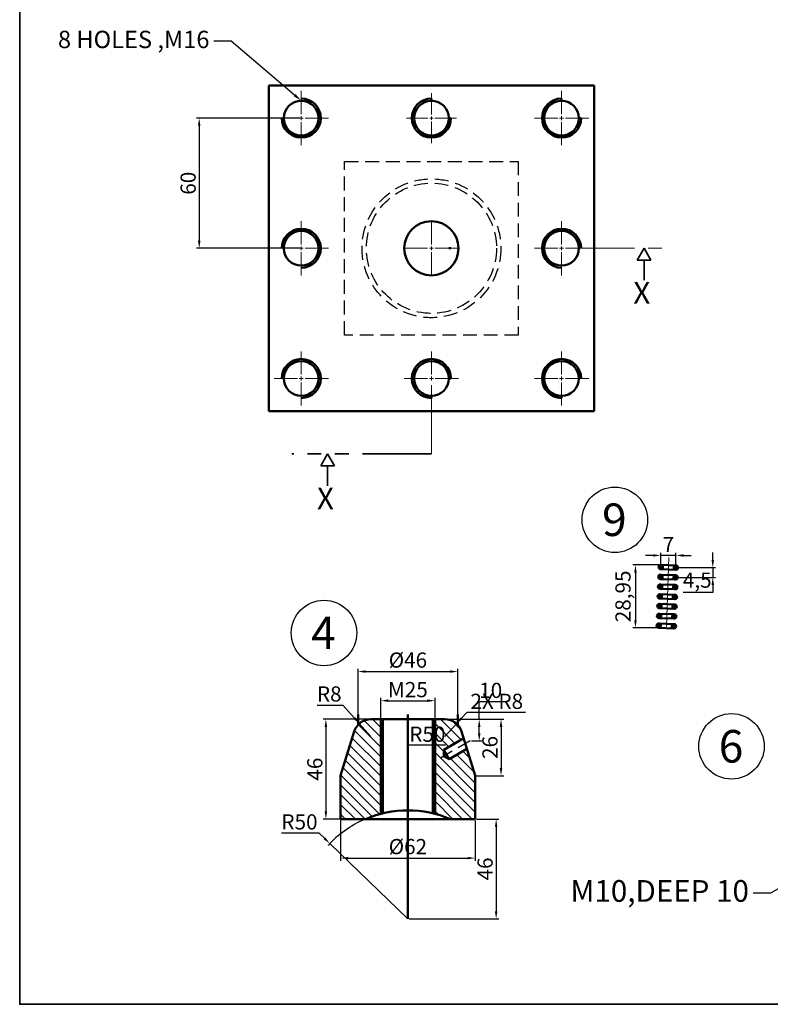
# Model space of a CAD drawing. Units: millimetres. Extents: x -5 to 1372, y -339 to 395.
# Tile 1 of 6: x -5 to 341, y -339 to 114. Entities that reach past the tile are written whole.
import ezdxf
from ezdxf import colors
from ezdxf.entities.mleader import LeaderData, LeaderLine
from ezdxf.math import Vec2, Vec3

# ---------------------------------------------------------------- set-up
doc = ezdxf.new("R2010")
doc.units = ezdxf.units.MM
for name, pattern in [('CENTER', [50.8, 31.75, -6.35, 6.35, -6.35]), ('HIDDEN', [9.525, 6.35, -3.175]), ('PHANTOM', [63.5, 31.75, -6.35, 6.35, -6.35, 6.35, -6.35])]:
    doc.linetypes.add(name, pattern=pattern)
for name, color, linetype, lineweight in [('M-CNTR', 1, 'CENTER', 18), ('M-DIMS', 2, 'Continuous', 25), ('M-HATC', 8, 'Continuous', 18), ('M-HIDN', 6, 'HIDDEN', 25), ('M-OUTL', 7, 'Continuous', 50), ('M-SECT', 4, 'PHANTOM', 35), ('M-TEXT', 3, 'Continuous', 25), ('M-TTLB', 7, 'Continuous', 35)]:
    doc.layers.add(name, color=color, linetype=linetype, lineweight=lineweight)
doc.styles.get("Standard").update_dxf_attribs({"font": 'arial.ttf'})
doc.dimstyles.new('ISO-25', dxfattribs={"dimtxt": 7, "dimasz": 3.5, "dimexe": 1.25, "dimexo": 0.625, "dimtad": 1, "dimtoh": 1, "dimtxsty": 'Standard', "dimcen": 2.5, "dimadec": 0, "dimazin": 0, "dimtfac": 1, "dimtmove": 0, "dimatfit": 3, "dimfxl": 1, "dimarcsym": 0})
pattern_1 = [(133, (-372.26105, -76.62878), (-0.2322048, -0.21653448), [])]
pattern_2 = [(133, (-372.4181, -81.12604), (-0.2322048, -0.21653448), [])]
pattern_3 = [(133, (-372.57515, -85.6233), (-0.2322048, -0.21653448), [])]
pattern_4 = [(133, (-372.7322, -90.12055), (-0.2322048, -0.21653448), [])]
pattern_5 = [(133, (-372.88924, -94.6178), (-0.2322048, -0.21653448), [])]
pattern_6 = [(133, (-373.0463, -99.11507), (-0.2322048, -0.21653448), [])]
pattern_7 = [(133, (-373.20334, -103.61233), (-0.2322048, -0.21653448), [])]

# ---------------------------------------------------------------- blocks, each defined once
blk = doc.blocks.new('*U17')
at = {"layer": 'M-CNTR', "color": 0, "transparency": 16777216}
for p, q in [((0, 1.8), (0, 12.5)), ((-12.5, 0), (-1.8, 0)), ((1.8, 0), (12.5, 0)), ((0, -12.5), (0, -1.8))]:
    blk.add_line(p, q, dxfattribs=at)
at = {"layer": 'M-CNTR', "color": 0, "linetype": 'Continuous', "transparency": 16777216}
for p, q in [((-0.9, 0), (0.9, 0)), ((0, -0.9), (0, 0.9))]:
    blk.add_line(p, q, dxfattribs=at)
blk = doc.blocks.new('*U18')
at = {"layer": 'M-CNTR', "color": 0, "transparency": 16777216}
for p, q in [((0, 1.8), (0, 12.5)), ((-12.5, 0), (-1.8, 0)), ((1.8, 0), (12.5, 0)), ((0, -34.79), (0, -1.8))]:
    blk.add_line(p, q, dxfattribs=at)
at = {"layer": 'M-CNTR', "color": 0, "linetype": 'Continuous', "transparency": 16777216}
for p, q in [((-0.9, 0), (0.9, 0)), ((0, -0.9), (0, 0.9))]:
    blk.add_line(p, q, dxfattribs=at)
blk = doc.blocks.new('*U19')
at = {"layer": 'M-CNTR', "color": 0, "transparency": 16777216}
for p, q in [((0, 1.8), (0, 12.5)), ((-12.5, 0), (-1.8, 0)), ((1.8, 0), (47.58, 0)), ((0, -12.5), (0, -1.8))]:
    blk.add_line(p, q, dxfattribs=at)
at = {"layer": 'M-CNTR', "color": 0, "linetype": 'Continuous', "transparency": 16777216}
for p, q in [((-0.9, 0), (0.9, 0)), ((0, -0.9), (0, 0.9))]:
    blk.add_line(p, q, dxfattribs=at)
blk = doc.blocks.new('*U20')
at = {"layer": 'M-CNTR', "color": 0, "transparency": 16777216}
for p, q in [((0, 1.8), (0, 12.5)), ((-12.5, 0), (-1.8, 0)), ((1.8, 0), (12.5, 0)), ((0, -12.5), (0, -1.8))]:
    blk.add_line(p, q, dxfattribs=at)
at = {"layer": 'M-CNTR', "color": 0, "linetype": 'Continuous', "transparency": 16777216}
for p, q in [((-0.9, 0), (0.9, 0)), ((0, -0.9), (0, 0.9))]:
    blk.add_line(p, q, dxfattribs=at)
blk = doc.blocks.new('*U21')
at = {"layer": 'M-CNTR', "color": 0, "transparency": 16777216}
for p, q in [((0, 1.8), (0, 12.5)), ((-12.5, 0), (-1.8, 0)), ((1.8, 0), (12.5, 0)), ((0, -12.5), (0, -1.8))]:
    blk.add_line(p, q, dxfattribs=at)
at = {"layer": 'M-CNTR', "color": 0, "linetype": 'Continuous', "transparency": 16777216}
for p, q in [((-0.9, 0), (0.9, 0)), ((0, -0.9), (0, 0.9))]:
    blk.add_line(p, q, dxfattribs=at)
blk = doc.blocks.new('*U22')
at = {"layer": 'M-CNTR', "color": 0, "transparency": 16777216}
for p, q in [((0, 1.8), (0, 12.5)), ((-12.5, 0), (-1.8, 0)), ((1.8, 0), (12.5, 0)), ((0, -12.5), (0, -1.8))]:
    blk.add_line(p, q, dxfattribs=at)
at = {"layer": 'M-CNTR', "color": 0, "linetype": 'Continuous', "transparency": 16777216}
for p, q in [((-0.9, 0), (0.9, 0)), ((0, -0.9), (0, 0.9))]:
    blk.add_line(p, q, dxfattribs=at)
blk = doc.blocks.new('*U23')
at = {"layer": 'M-CNTR', "color": 0, "transparency": 16777216}
for p, q in [((0, 1.6), (0, 11.5)), ((-11.5, 0), (-1.6, 0)), ((1.6, 0), (11.5, 0)), ((0, -11.5), (0, -1.6))]:
    blk.add_line(p, q, dxfattribs=at)
at = {"layer": 'M-CNTR', "color": 0, "linetype": 'Continuous', "transparency": 16777216}
for p, q in [((-0.8, 0), (0.8, 0)), ((0, -0.8), (0, 0.8))]:
    blk.add_line(p, q, dxfattribs=at)
blk = doc.blocks.new('*U24')
at = {"layer": 'M-CNTR', "color": 0, "transparency": 16777216}
for p, q in [((0, 1.8), (0, 12.5)), ((-12.5, 0), (-1.8, 0)), ((1.8, 0), (12.5, 0)), ((0, -12.5), (0, -1.8))]:
    blk.add_line(p, q, dxfattribs=at)
at = {"layer": 'M-CNTR', "color": 0, "linetype": 'Continuous', "transparency": 16777216}
for p, q in [((-0.9, 0), (0.9, 0)), ((0, -0.9), (0, 0.9))]:
    blk.add_line(p, q, dxfattribs=at)
blk = doc.blocks.new('*U25')
at = {"layer": 'M-CNTR', "color": 0, "transparency": 16777216}
for p, q in [((0, 1.8), (0, 12.5)), ((-12.5, 0), (-1.8, 0)), ((1.8, 0), (12.5, 0)), ((0, -12.5), (0, -1.8))]:
    blk.add_line(p, q, dxfattribs=at)
at = {"layer": 'M-CNTR', "color": 0, "linetype": 'Continuous', "transparency": 16777216}
for p, q in [((-0.9, 0), (0.9, 0)), ((0, -0.9), (0, 0.9))]:
    blk.add_line(p, q, dxfattribs=at)
blk = doc.blocks.new('*D26')
at = {"layer": 'Defpoints', "color": 0, "transparency": 16777216}
for p in [(124.85, 69.06), (77.81, 9.06), (124.85, 9.06)]:
    blk.add_point(p, dxfattribs=at)
at = {"layer": 'M-DIMS', "color": 0, "lineweight": -2, "transparency": 16777216}
for p, q in [((124.23, 69.06), (76.56, 69.06)), ((77.81, 65.56), (77.81, 12.56)), ((124.23, 9.06), (76.56, 9.06))]:
    blk.add_line(p, q, dxfattribs=at)
at = {"layer": 'M-DIMS', "color": 0, "transparency": 16777216}
for points in [[(77.22, 65.56), (78.39, 65.56), (77.81, 69.06)], [(77.22, 12.56), (78.39, 12.56), (77.81, 9.06)]]:
    blk.add_solid(points, dxfattribs=at)
at = {"layer": 'M-DIMS', "color": 0, "transparency": 16777216, "insert": (73.61, 39.06), "char_height": 7, "attachment_point": 5, "rotation": 90}
blk.add_mtext('60', dxfattribs=at)
blk = doc.blocks.new('*D68')
at = {"layer": 'Defpoints', "color": 0, "transparency": 16777216}
for p in [(138.04, -265.26), (174.01, -299.99)]:
    blk.add_point(p, dxfattribs=at)
at = {"layer": 'M-DIMS', "color": 0, "lineweight": -2, "transparency": 16777216}
for p, q in [((115.68, -260.4), (133, -260.4)), ((133, -260.4), (135.52, -262.83)), ((174.01, -299.99), (138.04, -265.26))]:
    blk.add_line(p, q, dxfattribs=at)
blk.add_arc((174.01, -299.99), 50, 113.7901, 137.4421, dxfattribs=at)
at = {"layer": 'M-DIMS', "color": 0, "transparency": 16777216}
blk.add_solid([(135.93, -262.41), (135.12, -263.25), (138.04, -265.26)], dxfattribs=at)
at = {"layer": 'M-DIMS', "color": 0, "transparency": 16777216, "insert": (124.03, -256.2), "char_height": 7, "attachment_point": 5}
blk.add_mtext('R50', dxfattribs=at)
blk = doc.blocks.new('*D69')
at = {"layer": 'Defpoints', "color": 0, "transparency": 16777216}
for p in [(156.92, -207.99), (136.21, -253.99), (154.42, -253.99)]:
    blk.add_point(p, dxfattribs=at)
at = {"layer": 'M-DIMS', "color": 0, "lineweight": -2, "transparency": 16777216}
for p, q in [((156.3, -207.99), (134.96, -207.99)), ((136.21, -211.49), (136.21, -250.49)), ((153.79, -253.99), (134.96, -253.99))]:
    blk.add_line(p, q, dxfattribs=at)
at = {"layer": 'M-DIMS', "color": 0, "transparency": 16777216}
for points in [[(135.62, -211.49), (136.79, -211.49), (136.21, -207.99)], [(135.62, -250.49), (136.79, -250.49), (136.21, -253.99)]]:
    blk.add_solid(points, dxfattribs=at)
at = {"layer": 'M-DIMS', "color": 0, "transparency": 16777216, "insert": (132.01, -230.99), "char_height": 7, "attachment_point": 5, "rotation": 90}
blk.add_mtext('46', dxfattribs=at)
blk = doc.blocks.new('*D70')
at = {"layer": 'Defpoints', "color": 0, "transparency": 16777216}
for p in [(186.51, -199.43), (161.51, -207.99), (186.51, -207.99)]:
    blk.add_point(p, dxfattribs=at)
at = {"layer": 'M-DIMS', "color": 0, "lineweight": -2, "transparency": 16777216}
for p, q in [((161.51, -207.36), (161.51, -198.18)), ((165.01, -199.43), (183.01, -199.43)), ((186.51, -207.36), (186.51, -198.18))]:
    blk.add_line(p, q, dxfattribs=at)
at = {"layer": 'M-DIMS', "color": 0, "transparency": 16777216}
for points in [[(165.01, -198.84), (165.01, -200.01), (161.51, -199.43)], [(183.01, -198.84), (183.01, -200.01), (186.51, -199.43)]]:
    blk.add_solid(points, dxfattribs=at)
at = {"layer": 'M-DIMS', "color": 0, "transparency": 16777216, "insert": (174.01, -195.23), "char_height": 7, "attachment_point": 5}
blk.add_mtext('M25', dxfattribs=at)
blk = doc.blocks.new('*D71')
at = {"layer": 'Defpoints', "color": 0, "transparency": 16777216}
for p in [(191.1, -207.99), (205.01, -233.99), (216.94, -233.99)]:
    blk.add_point(p, dxfattribs=at)
at = {"layer": 'M-DIMS', "color": 0, "lineweight": -2, "transparency": 16777216}
for p, q in [((191.73, -207.99), (218.19, -207.99)), ((216.94, -211.49), (216.94, -230.49)), ((205.64, -233.99), (218.19, -233.99))]:
    blk.add_line(p, q, dxfattribs=at)
at = {"layer": 'M-DIMS', "color": 0, "transparency": 16777216}
for points in [[(216.35, -211.49), (217.52, -211.49), (216.94, -207.99)], [(216.35, -230.49), (217.52, -230.49), (216.94, -233.99)]]:
    blk.add_solid(points, dxfattribs=at)
at = {"layer": 'M-DIMS', "color": 0, "transparency": 16777216, "insert": (212.74, -220.99), "char_height": 7, "attachment_point": 5, "rotation": 90}
blk.add_mtext('26', dxfattribs=at)
blk = doc.blocks.new('*D72')
at = {"layer": 'Defpoints', "color": 0, "transparency": 16777216}
for p in [(202.74, -207.99), (202.74, -217.99), (206.89, -217.99)]:
    blk.add_point(p, dxfattribs=at)
at = {"layer": 'M-DIMS', "color": 0, "lineweight": -2, "transparency": 16777216}
for p, q in [((206.89, -207.99), (206.89, -199.79)), ((206.89, -199.79), (216.86, -199.79)), ((203.36, -207.99), (208.14, -207.99)), ((206.89, -214.49), (206.89, -211.49)), ((203.36, -217.99), (208.14, -217.99))]:
    blk.add_line(p, q, dxfattribs=at)
at = {"layer": 'M-DIMS', "color": 0, "transparency": 16777216}
for points in [[(206.3, -211.49), (207.47, -211.49), (206.89, -207.99)], [(206.3, -214.49), (207.47, -214.49), (206.89, -217.99)]]:
    blk.add_solid(points, dxfattribs=at)
at = {"layer": 'M-DIMS', "color": 0, "transparency": 16777216, "insert": (212.18, -195.59), "char_height": 7, "attachment_point": 5}
blk.add_mtext('10', dxfattribs=at)
blk = doc.blocks.new('*D73')
at = {"layer": 'Defpoints', "color": 0, "transparency": 16777216}
for p in [(143.01, -253.99), (205.01, -253.99), (205.01, -271.98)]:
    blk.add_point(p, dxfattribs=at)
at = {"layer": 'M-DIMS', "color": 0, "lineweight": -2, "transparency": 16777216}
for p, q in [((143.01, -254.61), (143.01, -273.23)), ((205.01, -254.61), (205.01, -273.23)), ((146.51, -271.98), (201.51, -271.98))]:
    blk.add_line(p, q, dxfattribs=at)
at = {"layer": 'M-DIMS', "color": 0, "transparency": 16777216}
for points in [[(146.51, -271.4), (146.51, -272.56), (143.01, -271.98)], [(201.51, -271.4), (201.51, -272.56), (205.01, -271.98)]]:
    blk.add_solid(points, dxfattribs=at)
at = {"layer": 'M-DIMS', "color": 0, "transparency": 16777216, "insert": (174.01, -267.58), "char_height": 7, "attachment_point": 5}
blk.add_mtext('%%C62', dxfattribs=at)
blk = doc.blocks.new('*D74')
at = {"layer": 'Defpoints', "color": 0, "transparency": 16777216}
for p in [(197.01, -186.01), (151.01, -207.99), (197.01, -207.99)]:
    blk.add_point(p, dxfattribs=at)
at = {"layer": 'M-DIMS', "color": 0, "lineweight": -2, "transparency": 16777216}
for p, q in [((151.01, -207.36), (151.01, -184.76)), ((154.51, -186.01), (193.51, -186.01)), ((197.01, -207.36), (197.01, -184.76))]:
    blk.add_line(p, q, dxfattribs=at)
at = {"layer": 'M-DIMS', "color": 0, "transparency": 16777216}
for points in [[(154.51, -185.42), (154.51, -186.59), (151.01, -186.01)], [(193.51, -185.42), (193.51, -186.59), (197.01, -186.01)]]:
    blk.add_solid(points, dxfattribs=at)
at = {"layer": 'M-DIMS', "color": 0, "transparency": 16777216, "insert": (174.01, -181.61), "char_height": 7, "attachment_point": 5}
blk.add_mtext('%%C46', dxfattribs=at)
blk = doc.blocks.new('*D75')
at = {"layer": 'Defpoints', "color": 0, "transparency": 16777216}
for p in [(151.62, -210), (156.92, -215.99)]:
    blk.add_point(p, dxfattribs=at)
at = {"layer": 'M-DIMS', "color": 0, "lineweight": -2, "transparency": 16777216}
for p, q in [((132.11, -201.43), (144.04, -201.43)), ((144.04, -201.43), (149.3, -207.37)), ((156.92, -215.99), (151.62, -210))]:
    blk.add_line(p, q, dxfattribs=at)
at = {"layer": 'M-DIMS', "color": 0, "transparency": 16777216}
blk.add_solid([(149.73, -206.99), (148.86, -207.76), (151.62, -210)], dxfattribs=at)
at = {"layer": 'M-DIMS', "color": 0, "transparency": 16777216, "insert": (137.76, -197.24), "char_height": 7, "attachment_point": 5}
blk.add_mtext('R8', dxfattribs=at)
blk = doc.blocks.new('*D76')
at = {"layer": 'Defpoints', "color": 0, "transparency": 16777216}
for p in [(205.01, -253.99), (174.01, -299.99), (214.69, -299.99)]:
    blk.add_point(p, dxfattribs=at)
at = {"layer": 'M-DIMS', "color": 0, "lineweight": -2, "transparency": 16777216}
for p, q in [((205.64, -253.99), (215.94, -253.99)), ((214.69, -257.49), (214.69, -296.49)), ((174.64, -299.99), (215.94, -299.99))]:
    blk.add_line(p, q, dxfattribs=at)
at = {"layer": 'M-DIMS', "color": 0, "transparency": 16777216}
for points in [[(214.11, -257.49), (215.27, -257.49), (214.69, -253.99)], [(214.11, -296.49), (215.27, -296.49), (214.69, -299.99)]]:
    blk.add_solid(points, dxfattribs=at)
at = {"layer": 'M-DIMS', "color": 0, "transparency": 16777216, "insert": (210.49, -276.99), "char_height": 7, "attachment_point": 5, "rotation": 90}
blk.add_mtext('46', dxfattribs=at)
blk = doc.blocks.new('*D87')
at = {"layer": 'Defpoints', "color": 0, "transparency": 16777216}
for p in [(290.59, -132.49), (290.59, -137.86), (297.59, -138.1)]:
    blk.add_point(p, dxfattribs=at)
at = {"layer": 'M-DIMS', "color": 0, "lineweight": -2, "transparency": 16777216}
for p, q in [((290.59, -137.24), (290.59, -131.24)), ((297.59, -137.48), (297.59, -131.24)), ((287.09, -132.49), (283.59, -132.49)), ((297.59, -132.49), (290.59, -132.49)), ((301.09, -132.49), (304.59, -132.49))]:
    blk.add_line(p, q, dxfattribs=at)
at = {"layer": 'M-DIMS', "color": 0, "transparency": 16777216}
for points in [[(287.09, -131.91), (287.09, -133.07), (290.59, -132.49)], [(301.09, -131.91), (301.09, -133.07), (297.59, -132.49)]]:
    blk.add_solid(points, dxfattribs=at)
at = {"layer": 'M-DIMS', "color": 0, "transparency": 16777216, "insert": (294.09, -128.37), "char_height": 7, "attachment_point": 5}
blk.add_mtext('7', dxfattribs=at)
blk = doc.blocks.new('*D88')
at = {"layer": 'Defpoints', "color": 0, "transparency": 16777216}
for p in [(297.59, -138.1), (297.43, -142.6), (314.55, -142.6)]:
    blk.add_point(p, dxfattribs=at)
at = {"layer": 'M-DIMS', "color": 0, "lineweight": -2, "transparency": 16777216}
for p, q in [((314.55, -134.6), (314.55, -131.1)), ((298.22, -138.1), (315.8, -138.1)), ((314.55, -138.1), (314.55, -142.6)), ((298.06, -142.6), (315.8, -142.6)), ((314.55, -149.6), (300.85, -149.6)), ((314.55, -146.1), (314.55, -149.6))]:
    blk.add_line(p, q, dxfattribs=at)
at = {"layer": 'M-DIMS', "color": 0, "transparency": 16777216}
for points in [[(313.97, -134.6), (315.13, -134.6), (314.55, -138.1)], [(313.97, -146.1), (315.13, -146.1), (314.55, -142.6)]]:
    blk.add_solid(points, dxfattribs=at)
at = {"layer": 'M-DIMS', "color": 0, "transparency": 16777216, "insert": (307.39, -144.78), "char_height": 7, "attachment_point": 5}
blk.add_mtext('4,5', dxfattribs=at)
blk = doc.blocks.new('*D89')
at = {"layer": 'Defpoints', "color": 0, "transparency": 16777216}
for p in [(290.36, -136.89), (278.91, -165.83), (289.35, -165.83)]:
    blk.add_point(p, dxfattribs=at)
at = {"layer": 'M-DIMS', "color": 0, "lineweight": -2, "transparency": 16777216}
for p, q in [((289.73, -136.89), (277.66, -136.89)), ((278.91, -140.39), (278.91, -162.33)), ((288.72, -165.83), (277.66, -165.83))]:
    blk.add_line(p, q, dxfattribs=at)
at = {"layer": 'M-DIMS', "color": 0, "transparency": 16777216}
for points in [[(278.32, -140.39), (279.49, -140.39), (278.91, -136.89)], [(278.32, -162.33), (279.49, -162.33), (278.91, -165.83)]]:
    blk.add_solid(points, dxfattribs=at)
at = {"layer": 'M-DIMS', "color": 0, "transparency": 16777216, "insert": (274.07, -151.36), "char_height": 7, "attachment_point": 5, "rotation": 90}
blk.add_mtext('28,95', dxfattribs=at)
blk = doc.blocks.new('SECTION-ARROW')
for p, q in [((3.14, 5.44), (0, 0)), ((3.14, 5.44), (6.28, 0)), ((0, 0), (6.28, 0))]:
    blk.add_line(p, q)
blk = doc.blocks.new('HOLE-TAPPED')
for p, q in [((9, 18), (9, 17)), ((18, 9), (17, 9))]:
    blk.add_line(p, q)
blk.add_circle((9, 9), 8)
blk.add_arc((9, 9), 9, 90, 0)
blk = doc.blocks.new('*D100')
at = {"layer": 'Defpoints', "color": 0, "transparency": 16777216}
for p in [(174.01, -249.99), (174.01, -299.99)]:
    blk.add_point(p, dxfattribs=at)
at = {"layer": 'M-DIMS', "color": 0, "lineweight": -2, "transparency": 16777216}
for p, q in [((191.34, -219.99), (174.01, -219.99)), ((174.01, -219.99), (174.01, -246.49)), ((174.01, -299.99), (174.01, -249.99))]:
    blk.add_line(p, q, dxfattribs=at)
at = {"layer": 'M-DIMS', "color": 0, "transparency": 16777216}
blk.add_solid([(173.43, -246.49), (174.6, -246.49), (174.01, -249.99)], dxfattribs=at)
at = {"layer": 'M-DIMS', "color": 0, "transparency": 16777216, "insert": (182.99, -215.79), "char_height": 7, "attachment_point": 5}
blk.add_mtext('R50', dxfattribs=at)
blk = doc.blocks.new('*D101')
at = {"layer": 'Defpoints', "color": 0, "transparency": 16777216}
for p in [(196.45, -210.03), (191.1, -215.99)]:
    blk.add_point(p, dxfattribs=at)
at = {"layer": 'M-DIMS', "color": 0, "lineweight": -2, "transparency": 16777216}
for p, q in [((201.13, -204.83), (198.79, -207.43)), ((228.21, -204.83), (201.13, -204.83)), ((191.1, -215.99), (196.45, -210.03))]:
    blk.add_line(p, q, dxfattribs=at)
at = {"layer": 'M-DIMS', "color": 0, "transparency": 16777216}
blk.add_solid([(198.35, -207.04), (199.22, -207.82), (196.45, -210.03)], dxfattribs=at)
at = {"layer": 'M-DIMS', "color": 0, "transparency": 16777216, "insert": (214.98, -200.63), "char_height": 7, "attachment_point": 5}
blk.add_mtext('2X R8', dxfattribs=at)

msp = doc.modelspace()

# ---------------------------------------------------------------- hatches: boundary and pattern name
at = {"layer": 'M-HATC'}
h = msp.add_hatch(dxfattribs=at)
h.set_pattern_fill('ANSI31', color=256, scale=0.1, angle=88)
h.set_pattern_definition(pattern_1)
h.paths.add_polyline_path([(291.594, -137.86, 1), (289.594, -137.86, 1)])
h = msp.add_hatch(dxfattribs=at)
h.set_pattern_fill('ANSI31', color=256, scale=0.1, angle=88)
h.set_pattern_definition(pattern_1)
h.paths.add_polyline_path([(298.59, -138.105, 1), (296.59, -138.105, 1)])
h = msp.add_hatch(dxfattribs=at)
h.set_pattern_fill('ANSI31', color=256, scale=0.1, angle=88)
h.set_pattern_definition(pattern_2)
h.paths.add_polyline_path([(291.437, -142.358, 1), (289.437, -142.358, 1)])
h = msp.add_hatch(dxfattribs=at)
h.set_pattern_fill('ANSI31', color=256, scale=0.1, angle=88)
h.set_pattern_definition(pattern_2)
h.paths.add_polyline_path([(298.433, -142.602, 1), (296.433, -142.602, 1)])
h = msp.add_hatch(dxfattribs=at)
h.set_pattern_fill('ANSI31', color=256, scale=0.1, angle=88)
h.set_pattern_definition(pattern_3)
h.paths.add_polyline_path([(291.28, -146.855, 1), (289.28, -146.855, 1)])
h = msp.add_hatch(dxfattribs=at)
h.set_pattern_fill('ANSI31', color=256, scale=0.1, angle=88)
h.set_pattern_definition(pattern_3)
h.paths.add_polyline_path([(298.276, -147.099, 1), (296.276, -147.099, 1)])
h = msp.add_hatch(dxfattribs=at)
h.set_pattern_fill('ANSI31', color=256, scale=0.1, angle=88)
h.set_pattern_definition(pattern_4)
h.paths.add_polyline_path([(291.123, -151.352, 1), (289.123, -151.352, 1)])
h = msp.add_hatch(dxfattribs=at)
h.set_pattern_fill('ANSI31', color=256, scale=0.1, angle=88)
h.set_pattern_definition(pattern_4)
h.paths.add_polyline_path([(298.119, -151.596, 1), (296.119, -151.596, 1)])
h = msp.add_hatch(dxfattribs=at)
h.set_pattern_fill('ANSI31', color=256, scale=0.1, angle=88)
h.set_pattern_definition(pattern_5)
h.paths.add_polyline_path([(290.966, -155.849, 1), (288.966, -155.849, 1)])
h = msp.add_hatch(dxfattribs=at)
h.set_pattern_fill('ANSI31', color=256, scale=0.1, angle=88)
h.set_pattern_definition(pattern_5)
h.paths.add_polyline_path([(297.962, -156.094, 1), (295.962, -156.094, 1)])
h = msp.add_hatch(dxfattribs=at)
h.set_pattern_fill('ANSI31', color=256, scale=0.1, angle=88)
h.set_pattern_definition(pattern_6)
h.paths.add_polyline_path([(290.809, -160.347, 1), (288.809, -160.347, 1)])
h = msp.add_hatch(dxfattribs=at)
h.set_pattern_fill('ANSI31', color=256, scale=0.1, angle=88)
h.set_pattern_definition(pattern_6)
h.paths.add_polyline_path([(297.805, -160.591, 1), (295.805, -160.591, 1)])
h = msp.add_hatch(dxfattribs=at)
h.set_pattern_fill('ANSI31', color=256, scale=0.1, angle=88)
h.set_pattern_definition(pattern_7)
h.paths.add_polyline_path([(290.652, -164.844, 1), (288.652, -164.844, 1)])
h = msp.add_hatch(dxfattribs=at)
h.set_pattern_fill('ANSI31', color=256, scale=0.1, angle=88)
h.set_pattern_definition(pattern_7)
h.paths.add_polyline_path([(297.648, -165.088, 1), (295.648, -165.088, 1)])
h = msp.add_hatch(dxfattribs=at)
h.set_pattern_fill('ANSI31', color=256, angle=90)
h.set_pattern_definition([(135, (-770.229, -407.1155), (-2.245064, -2.245064), [])])
h.paths.add_polyline_path([(161.512, -207.985), (156.921, -207.985, 0.3292536), (149.274, -213.633), (143.012, -233.985), (143.012, -253.985), (154.416, -253.985, -0.0375265), (161.512, -251.573)])
h.paths.add_polyline_path([(186.512, -251.573, -0.0375265), (193.608, -253.985), (205.012, -253.985), (205.012, -233.985), (201.226, -221.682), (193.062, -226.396), (190.562, -224.953), (190.562, -222.066), (199.718, -216.779), (198.75, -213.633, 0.3292536), (191.103, -207.985), (186.512, -207.985)])

# ---------------------------------------------------------------- linework, layer by layer
at = {"layer": 'M-CNTR'}
msp.add_line((294.249, -133.497), (293.08, -166.965), dxfattribs=at)
at = {"layer": 'M-HIDN'}
msp.add_line((202.737, -217.923), (188.701, -226.027), dxfattribs=at)
msp.add_lwpolyline([(144.854, 49.065), (224.854, 49.065), (224.854, -30.935), (144.854, -30.935)], close=True, dxfattribs=at)
for radius in [32, 30]:
    msp.add_circle((184.854, 9.065), radius, dxfattribs=at)
at = {"layer": 'M-OUTL'}
for p, q in [((109.854, 84.065), (259.854, 84.065)), ((109.854, -65.935), (109.854, 84.065)), ((259.854, 84.065), (259.854, -65.935)), ((193.854, 9.065), (192.854, 9.065)), ((244.854, -59.935), (244.854, -58.935)), ((259.854, -65.935), (109.854, -65.935)), ((290.559, -138.86), (297.555, -139.104)), ((290.629, -136.861), (297.625, -137.105)), ((290.402, -143.357), (297.398, -143.601)), ((290.472, -141.358), (297.468, -141.603)), ((290.245, -147.854), (297.241, -148.099)), ((290.315, -145.856), (297.311, -146.1)), ((290.088, -152.352), (297.084, -152.596)), ((290.158, -150.353), (297.154, -150.597)), ((289.931, -156.849), (296.927, -157.093)), ((290.001, -154.85), (296.997, -155.094)), ((289.774, -161.346), (296.77, -161.59)), ((289.844, -159.347), (296.84, -159.592)), ((289.617, -165.843), (296.613, -166.088)), ((289.687, -163.845), (296.683, -164.089)), ((151.012, -210.592), (151.012, -205.725)), ((191.103, -207.985), (156.921, -207.985)), ((161.512, -207.985), (161.512, -251.573)), ((162.512, -207.985), (162.512, -251.326)), ((174.012, -207.985), (174.012, -205.725)), ((174.012, -207.985), (174.012, -299.985)), ((185.512, -207.985), (185.512, -251.326)), ((186.512, -207.985), (186.512, -251.573)), ((197.012, -210.592), (197.012, -205.725)), ((149.274, -213.633), (143.012, -233.985)), ((199.718, -216.779), (190.562, -222.066)), ((198.75, -213.633), (205.012, -233.985)), ((190.562, -222.066), (193.062, -226.396)), ((190.562, -222.066), (190.562, -224.953)), ((201.226, -221.682), (193.062, -226.396)), ((193.062, -226.396), (190.562, -224.953)), ((143.012, -233.985), (143.012, -253.985)), ((205.012, -253.985), (205.012, -233.985)), ((143.012, -253.985), (205.012, -253.985))]:
    msp.add_line(p, q, dxfattribs=at)
for centre, radius in [((124.854, 69.065), 8), ((184.854, 9.065), 12.5), ((124.854, 9.065), 8), ((244.854, 9.065), 8), ((124.854, -50.935), 8), ((244.854, -50.935), 8), ((290.594, -137.86), 1), ((297.59, -138.105), 1), ((290.437, -142.358), 1), ((297.433, -142.602), 1), ((290.28, -146.855), 1), ((297.276, -147.099), 1), ((290.123, -151.352), 1), ((297.119, -151.596), 1), ((289.966, -155.849), 1), ((296.962, -156.094), 1), ((289.809, -160.347), 1), ((296.805, -160.591), 1), ((289.652, -164.844), 1), ((296.648, -165.088), 1)]:
    msp.add_circle(centre, radius, dxfattribs=at)
for centre, radius, start, end in [((124.854, 69.065), 9, 180, 90), ((124.854, 9.065), 9, 270, 180), ((244.854, 9.065), 9, 0, 270), ((124.854, -50.935), 9, 270, 180), ((244.854, -50.935), 9, 0, 270), ((156.921, -215.985), 8, 90, 162.89727), ((191.103, -215.985), 8, 17.10273, 90), ((174.012, -299.985), 50, 66.92608, 113.07392)]:
    msp.add_arc(centre, radius, start, end, dxfattribs=at)
at = {"layer": 'M-SECT'}
for p, q in [((282.845, 3.628), (282.845, -5.56)), ((184.854, -85.72), (120.439, -85.72)), ((137.007, -91.157), (137.007, -100.346))]:
    msp.add_line(p, q, dxfattribs=at)
at = {"layer": 'M-TEXT'}
for centre in [(269.407, -116.069), (135.326, -168.216), (323.177, -220.485)]:
    msp.add_circle(centre, 15.085, dxfattribs=at)
at = {"layer": 'M-TTLB'}
msp.add_lwpolyline([(-4.944, 394.729), (1371.917, 394.729), (1371.917, -339.365), (-4.944, -339.365)], close=True, dxfattribs=at)

# ---------------------------------------------------------------- block references
at = {"layer": 'M-CNTR'}
for name, p in [('*U22', (124.854, 69.065)), ('*U23', (184.854, 69.065)), ('*U24', (244.854, 69.065)), ('*U21', (124.854, 9.065)), ('*U20', (184.854, 9.065)), ('*U19', (244.854, 9.065)), ('*U25', (124.854, -50.935)), ('*U18', (184.854, -50.935)), ('*U17', (244.854, -50.935))]:
    msp.add_blockref(name, p, dxfattribs=at)
at = {"layer": 'M-OUTL'}
for p in [(175.854, 60.065), (235.854, 60.065)]:
    msp.add_blockref('HOLE-TAPPED', p, dxfattribs=at)
at = {"layer": 'M-OUTL', "rotation": 270.0000000000002}
msp.add_blockref('HOLE-TAPPED', (175.854, -41.935), dxfattribs=at)
at = {"layer": 'M-SECT', "rotation": 120.0000000000006}
msp.add_blockref('SECTION-ARROW', (285.983, 3.629), dxfattribs=at)
at = {"layer": 'M-SECT'}
msp.add_blockref('SECTION-ARROW', (133.869, -91.157), dxfattribs=at)

# ---------------------------------------------------------------- texts
at = {"layer": 'M-TEXT', "attachment_point": 1}
for s, width, insert, char_height in [('X', 15.979, (277.922, -6.445), 10), ('X', 15.979, (132.085, -101.23), 10), ('9', 15, (263.512, -108.538), 15), ('4', 15, (129.431, -160.685), 15), ('6', 15, (317.282, -212.954), 15)]:
    msp.add_mtext_dynamic_manual_height_columns(s, width=width, gutter_width=12.5, heights=[0], dxfattribs=dict(at, insert=insert, char_height=char_height))

# ---------------------------------------------------------------- dimensions: what is measured, and where the dimension line sits
at = {"layer": 'M-DIMS'}
for base, p1, p2, picture, middle in [((77.808, 9.065), (124.854, 69.065), (124.854, 9.065), '*D26', (73.609, 39.065)), ((314.55, -142.602), (297.59, -138.105), (297.433, -142.602), '*D88', (307.386, -144.785)), ((278.906, -165.834), (290.36, -136.888), (289.349, -165.834), '*D89', (274.075, -151.361)), ((136.205, -253.985), (156.921, -207.985), (154.416, -253.985), '*D69', (132.006, -230.985)), ((216.937, -233.985), (191.103, -207.985), (205.012, -233.985), '*D71', (212.738, -220.985)), ((214.689, -299.985), (205.012, -253.985), (174.012, -299.985), '*D76', (210.49, -276.985))]:
    dim = msp.add_linear_dim(base=base, p1=p1, p2=p2, angle=90, dimstyle='ISO-25', override={"dimclrd": 0, "dimclre": 0, "dimclrt": 0}, dxfattribs=at)
    dim.commit()
    dim.dimension.update_dxf_attribs({"geometry": picture, "text_midpoint": middle})
dim = msp.add_linear_dim(base=(290.594, -132.491), p1=(297.59, -138.105), p2=(290.594, -137.86), dimstyle='ISO-25', override={"dimclrd": 0, "dimclre": 0, "dimclrt": 0}, dxfattribs=at)
dim.commit()
dim.dimension.update_dxf_attribs({"geometry": '*D87', "text_midpoint": (294.092, -128.366)})
for base, p1, p2, text, picture, middle in [((197.012, -186.008), (151.012, -207.985), (197.012, -207.985), '%%C<>', '*D74', (174.012, -181.613)), ((186.512, -199.428), (161.512, -207.985), (186.512, -207.985), 'M<>', '*D70', (174.012, -195.229)), ((205.012, -271.979), (143.012, -253.985), (205.012, -253.985), '%%C<>', '*D73', (174.012, -267.584))]:
    dim = msp.add_linear_dim(base=base, p1=p1, p2=p2, text=text, dimstyle='ISO-25', override={"dimclrd": 0, "dimclre": 0, "dimclrt": 0}, dxfattribs=at)
    dim.commit()
    dim.dimension.update_dxf_attribs({"geometry": picture, "text_midpoint": middle})
dim = msp.add_radius_dim(center=(191.103, -215.985), mpoint=(196.449, -210.034), text='2X <>', dimstyle='ISO-25', override={"dimdec": 0, "dimlfac": 1, "dimrnd": 0, "dimzin": 0, "dimdsep": 46, "dimlunit": 2}, dxfattribs=at)
dim.commit()
dim.dimension.update_dxf_attribs({"geometry": '*D101', "text_midpoint": (214.983, -200.627)})
for center, mpoint, override, picture, middle in [((156.921, -215.985), (151.618, -209.995), {"dimclrd": 0, "dimclre": 0, "dimclrt": 0}, '*D75', (137.764, -201.435)), ((174.012, -299.985), (174.012, -249.985), {"dimdec": 0, "dimlfac": 1, "dimrnd": 0, "dimzin": 0, "dimdsep": 46, "dimlunit": 2}, '*D100', (182.988, -219.985))]:
    dim = msp.add_radius_dim(center=center, mpoint=mpoint, dimstyle='ISO-25', override=override, dxfattribs=at)
    dim.commit()
    dim.dimension.update_dxf_attribs({"geometry": picture, "text_midpoint": middle, "dimtype": 164})
dim = msp.add_linear_dim(base=(206.888, -217.985), p1=(202.737, -207.985), p2=(202.737, -217.985), angle=90, dimstyle='ISO-25', override={"dimclrd": 0, "dimclre": 0, "dimclrt": 0}, dxfattribs=at)
dim.commit()
dim.dimension.update_dxf_attribs({"geometry": '*D72', "text_midpoint": (212.185, -199.787), "dimtype": 160})
dim = msp.add_radius_dim(center=(174.012, -299.985), mpoint=(138.039, -265.258), dimstyle='ISO-25', override={"dimclrd": 0, "dimclre": 0, "dimclrt": 0}, dxfattribs=at)
dim.commit()
dim.dimension.update_dxf_attribs({"geometry": '*D68', "text_midpoint": (124.027, -256.198)})

# ---------------------------------------------------------------- leaders
ml = msp.add_multileader_mtext('Standard', dxfattribs=at)
ml.set_content('8 HOLES ,M16', color=256)
ml.set_leader_properties()
ml.build(insert=Vec2(0, 0))
ctx = ml.context
ctx.base_point, ctx.char_height, ctx.plane_origin = Vec3(6.354, 104.53), 8, Vec3(124.854, 77.065)
ctx.text_align_type = 2
notes = []
notes.append((ctx, [(0, (1, 1, 0), (92.547, 104.53), (-1, 0), 8, [(0, [(124.854, 77.065)], 0, [])])]))
ctx.mtext.insert, ctx.mtext.alignment, ctx.mtext.flow_direction = Vec3(82.547, 109.321), 3, 5
ml = msp.add_multileader_mtext('Standard', dxfattribs=at)
ml.set_content('M10,DEEP 10', color=256)
ml.set_leader_properties()
ml.build(insert=Vec2(0, 0))
ctx = ml.context
ctx.base_point, ctx.char_height, ctx.plane_origin = Vec3(242.403, -288.108), 10, Vec3(363.875, -275.027)
ctx.text_align_type = 2
notes.append((ctx, [(0, (1, 1, 0), (341.217, -288.108), (-1, 0), 8, [(0, [(363.875, -275.027)], 0, [])])]))
ctx.mtext.insert, ctx.mtext.alignment, ctx.mtext.flow_direction = Vec3(331.217, -282.119), 3, 5
for ctx, leaders in notes:
    for number, flags, end, landing, length, lines in leaders:
        leader = LeaderData()
        leader.index, (leader.has_last_leader_line, leader.has_dogleg_vector, leader.attachment_direction) = number, flags
        leader.last_leader_point, leader.dogleg_vector, leader.dogleg_length = Vec3(end), Vec3(landing), length
        for number, points, colour, breaks in lines:
            line = LeaderLine()
            line.index, line.vertices, line.color, line.breaks = number, Vec3.list(points), colors.encode_raw_color(colour), breaks
            leader.lines.append(line)
        ctx.leaders.append(leader)

doc.saveas('drawing.dxf')
